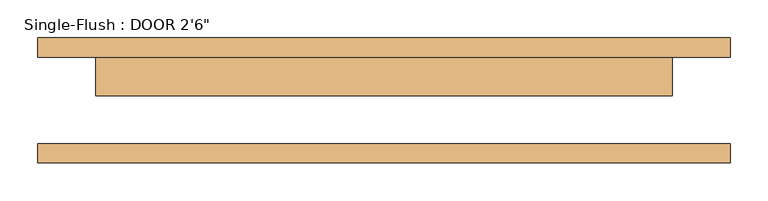
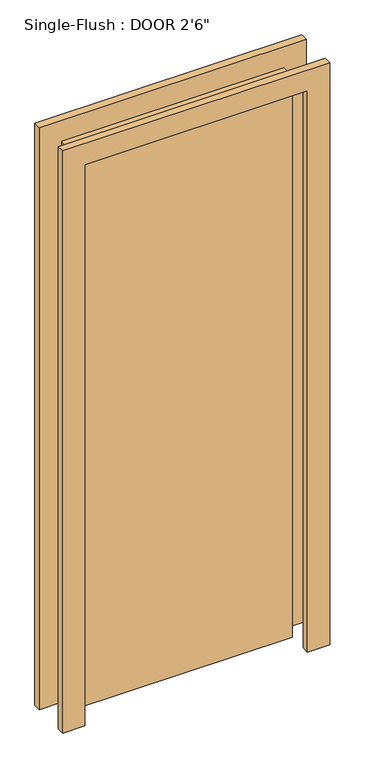
"""IFC4 building model written with IfcOpenShell, lengths in millimetres: door geometry."""

from ifc_helpers import new_model, si_unit, frame, origin, origin_with_axes, place, context, project, spatial, polyline, outline, extrude, source, transform, mapped, element, save


def door_d8f5dbb5(model_context):
    return source(origin(), model_context, "Body", "SweptSolid", [
        extrude(outline(polyline([(2108.2, -457.2), (0.0, -457.2), (0.0, -381.0), (2032.0, -381.0), (2032.0, 381.0), (0.0, 381.0), (0.0, 457.2), (2108.2, 457.2), (2108.2, -457.2)])), frame((0.0, 57.15, 0.0), z_axis=(0.0, 1.0, 0.0), x_axis=(0.0, 0.0, 1.0)), (0.0, 0.0, 1.0), 25.4),
        extrude(outline(polyline([(2108.2, 457.2), (2108.2, -457.2), (0.0, -457.2), (0.0, -381.0), (2032.0, -381.0), (2032.0, 381.0), (0.0, 381.0), (0.0, 457.2), (2108.2, 457.2)])), frame((0.0, -82.55, 0.0), z_axis=(0.0, 1.0, 0.0), x_axis=(0.0, 0.0, 1.0)), (0.0, 0.0, 1.0), 25.4),
        extrude(outline(polyline([(381.0, 6.35), (-381.0, 6.35), (-381.0, 57.15), (381.0, 57.15), (381.0, 6.35)])), origin_with_axes(), (0.0, 0.0, 1.0), 2032.0),
    ])


if __name__ == "__main__":
    model = new_model("IFC4")
    model_context = context("Model", 3, world=origin())
    ifc_project = project(units=[si_unit("LENGTHUNIT", "METRE", prefix="MILLI")], contexts=[model_context])
    site = spatial("IfcSite", under=ifc_project)
    building = spatial("IfcBuilding", under=site)
    placement = place(None, origin())
    door_shape = door_d8f5dbb5(model_context)
    element("IfcDoor", 1, ObjectType="Single-Flush : DOOR 2'6\"", at=placement, inside=building, context=model_context, shape_type="MappedRepresentation", body=[
        mapped(door_shape, transform((0.0, 0.0, 0.0), x_axis=(1.0, 0.0, 0.0), y_axis=(0.0, 1.0, 0.0), z_axis=(0.0, 0.0, 1.0))),
    ])
    save(model, "model.ifc")

# Revit data of these elements
# Type "Single-Flush : DOOR 2'6\""
#   Type Mark = "9"
#   Construction Type Id = "MDOOR"
#   Assembly Code = "C1020"
#   Analytic Construction = "Metal"
#   Thickness = 0' - 2"
#   Heat Transfer Coefficient (U) = 0.651978 BTU/(h·ft²·°F)
#   Height = 6' - 8"
#   Trim Projection Ext = 0' - 1"
#   Trim Projection Int = 0' - 1"
#   Trim Width = 0' - 3"
#   Width = 2' - 6"
#   Define Thermal Properties by = 1
#   Door Material = Door - Panel
#   Frame Material = Door - Frame
#   Visual Light Transmittance = 0
#   Solar Heat Gain Coefficient = 0
#   Function = (empty or 0)
#   Wall Closure = (empty or 0)
# Element 1 (IfcDoor, "Single-Flush : DOOR 2'6\"")
#   Materials on its faces: "Door - Frame", "Door - Panel"
# Materials
#   "Door - Panel": class "Wood", colour RGB 210 159 95, transparency 0, Cost = 0
#   "Door - Frame": colour RGB 118 70 51, transparency 0, Cost = 0
